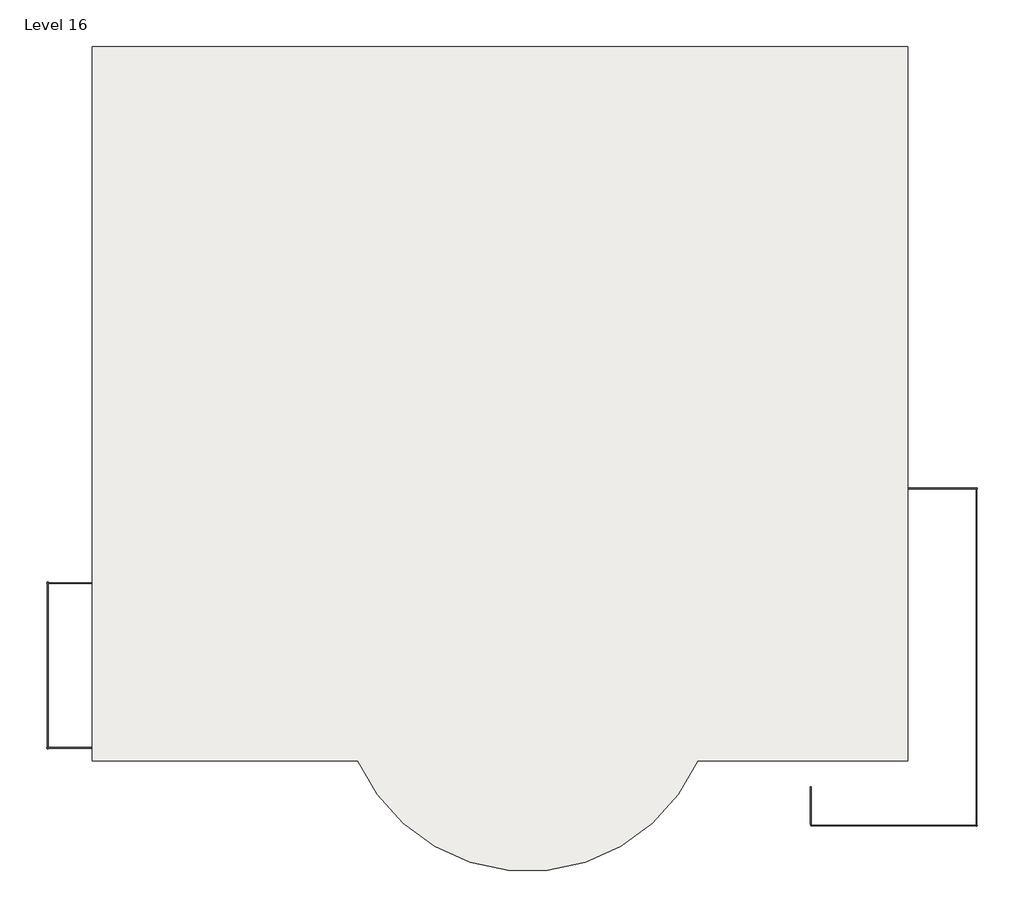
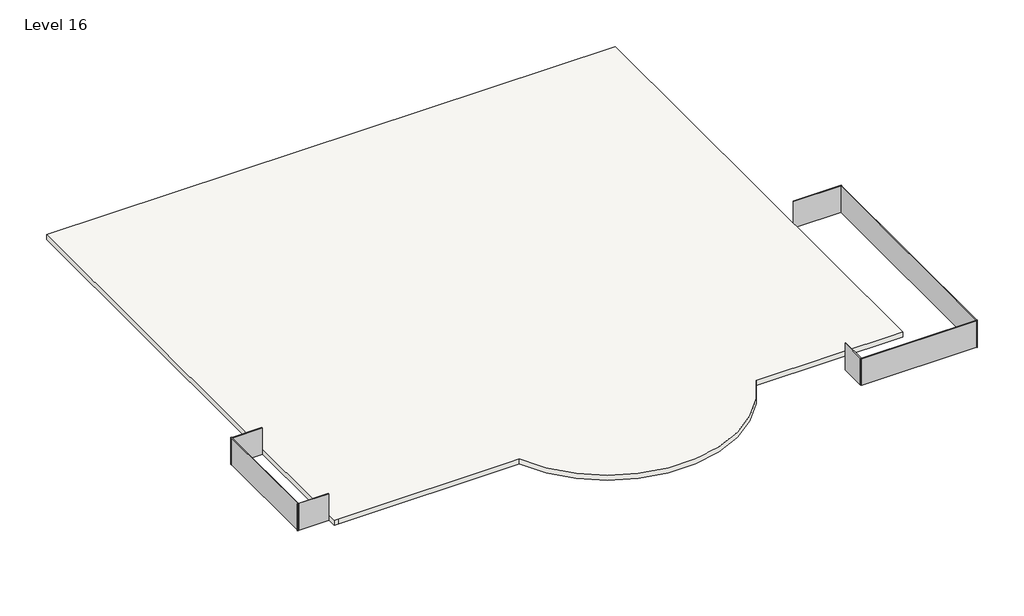
# One storey: 7 plates, 1 slab.
"""IFC4 building model written with IfcOpenShell, lengths in millimetres."""

from ifc_helpers import new_model, si_unit, point, frame, frame_2d, origin, place, context, project, spatial, polyline, circle_curve, trimmed, segment, composite_curve, outline, extrude, transform, mapped, element, save
from components import system_panel_glazed_7d767388, system_panel_glazed_c55d8a5b, system_panel_glazed_6865593f, system_panel_glazed_cbb493b5, system_panel_glazed_c4c31c98

model = new_model("IFC4")

# Units and contexts
model_context = context("Model", 3, world=origin())
ifc_project = project(units=[si_unit("LENGTHUNIT", "METRE", prefix="MILLI")], contexts=[model_context])

# Site, building, storey
site = spatial("IfcSite", under=ifc_project)
building = spatial("IfcBuilding", under=site)
storey = spatial("IfcBuildingStorey", under=building, Name="Level 16", Elevation=25984.2)

# Plates
placement = place(None, origin())
system_panel_glazed_shape = system_panel_glazed_7d767388(model_context)
element("IfcPlate", 1, ObjectType="System Panel : Glazed", at=placement, inside=storey, context=model_context, shape_type="MappedRepresentation", body=[
    mapped(system_panel_glazed_shape, transform((-17306.4505427, -8690.0239591, 25984.2), x_axis=(-1.0, 0.0, 0.0), y_axis=(0.0, -1.0, 0.0), z_axis=(0.0, 0.0, 1.0))),
])
element("IfcPlate", 2, ObjectType="System Panel : Glazed", at=placement, inside=storey, context=model_context, shape_type="MappedRepresentation", body=[
    mapped(system_panel_glazed_shape, transform((-17306.4505427, -13719.2239591, 25984.2), x_axis=(1.0, 0.0, 0.0), y_axis=(0.0, 1.0, 0.0), z_axis=(0.0, 0.0, 1.0))),
])
system_panel_glazed_2_shape = system_panel_glazed_c55d8a5b(model_context)
element("IfcPlate", 3, ObjectType="System Panel : Glazed", at=placement, inside=storey, context=model_context, shape_type="MappedRepresentation", body=[
    mapped(system_panel_glazed_2_shape, transform((-17979.5505427, -11204.6239591, 25984.2), x_axis=(0.0, -1.0, 0.0), y_axis=(1.0, 0.0, 0.0), z_axis=(0.0, 0.0, 1.0))),
])
element("IfcPlate", 4, ObjectType="System Panel : Glazed", at=placement, inside=storey, context=model_context, shape_type="MappedRepresentation", body=[
    mapped(system_panel_glazed_2_shape, transform((7561.1618272, -15995.7808221, 25984.2), x_axis=(-1.0, 0.0, 0.0), y_axis=(0.0, -1.0, 0.0), z_axis=(0.0, 0.0, 1.0))),
])
system_panel_glazed_3_shape = system_panel_glazed_6865593f(model_context)
element("IfcPlate", 5, ObjectType="System Panel : Glazed", at=placement, inside=storey, context=model_context, shape_type="MappedRepresentation", body=[
    mapped(system_panel_glazed_3_shape, transform((9033.0791312, -5892.9308221, 25984.2), x_axis=(1.0, 0.0, 0.0), y_axis=(0.0, 1.0, 0.0), z_axis=(0.0, 0.0, 1.0))),
])
system_panel_glazed_4_shape = system_panel_glazed_cbb493b5(model_context)
element("IfcPlate", 6, ObjectType="System Panel : Glazed", at=placement, inside=storey, context=model_context, shape_type="MappedRepresentation", body=[
    mapped(system_panel_glazed_4_shape, transform((10016.0464352, -10976.1058221, 25984.2), x_axis=(0.0, -1.0, 0.0), y_axis=(1.0, 0.0, 0.0), z_axis=(0.0, 0.0, 1.0))),
])
system_panel_glazed_5_shape = system_panel_glazed_c4c31c98(model_context)
element("IfcPlate", 7, ObjectType="System Panel : Glazed", at=placement, inside=storey, context=model_context, shape_type="MappedRepresentation", body=[
    mapped(system_panel_glazed_5_shape, transform((5088.4464352, -15426.9793258, 25984.2), x_axis=(0.0, 1.0, 0.0), y_axis=(-1.0, 0.0, 0.0), z_axis=(0.0, 0.0, 1.0))),
])

# Slab
element("IfcSlab", 8, ObjectType="9\"", at=placement, inside=storey, context=model_context, shape_type="SweptSolid", body=[
    extrude(outline(composite_curve([segment(polyline([(-16607.9505427, 7461.1191779), (7979.2494573, 7461.1191779), (7979.2494573, -14078.0808221), (1652.8739931, -14078.0808221)]), True, "CONTINUOUS"), segment(trimmed(circle_curve(frame_2d((-3476.1505427, -11788.3650223)), 5616.9111737), [point((1652.8739931, -14078.0808221))], [point((-8605.1750786, -14078.0808221))], False, "CARTESIAN"), True, "CONTINUOUS"), segment(polyline([(-8605.1750786, -14078.0808221), (-16404.7505427, -14078.0808221), (-16607.9505427, -14078.0808221), (-16607.9505427, 7461.1191779)]), True, "CONTINUOUS")], self_intersect=False)), frame((0.0, 0.0, 25984.2), z_axis=(0.0, 0.0, 1.0), x_axis=(1.0, 0.0, 0.0)), (0.0, 0.0, 1.0), 228.6),
])

save(model, "model.ifc")

# Revit data of these elements
# Type "System Panel : Glazed"
#   Construction Type Id = "GSP4R"
#   Analytic Construction = "1/8 in Pilkington single glazing"
#   Visual Light Transmittance = 0.9
#   Solar Heat Gain Coefficient = 0.86
#   Heat Transfer Coefficient (U) = 1.18115 BTU/(h·ft²·°F)
# Type "9\""
#   Assembly Code = "B1010"
#   Function = 0
#   Layers, outside or top first: 0' - 9" no material (function 1)
# Elements 1, 2, 3, 4, 5, 6, 7 (IfcPlate, "System Panel : Glazed")
#   Phase Created = New Construction
#   Materials on its faces: "Glass"
# Element 8 (IfcSlab, "9\"")
#   built-in parameter 1001955 = 1.5708 (stored number, unit not read)
#   Height Offset From Level = 0' - 9"
#   Phase Created = New Construction
#   Materials on its faces: "Default Floor"
# Materials
#   "Glass": class "Glass", colour RGB 0 128 192, transparency 0.75, Description = "Soda Lime Glass", Cost = 0
#   "Default Floor": colour RGB 128 128 128, transparency 0
